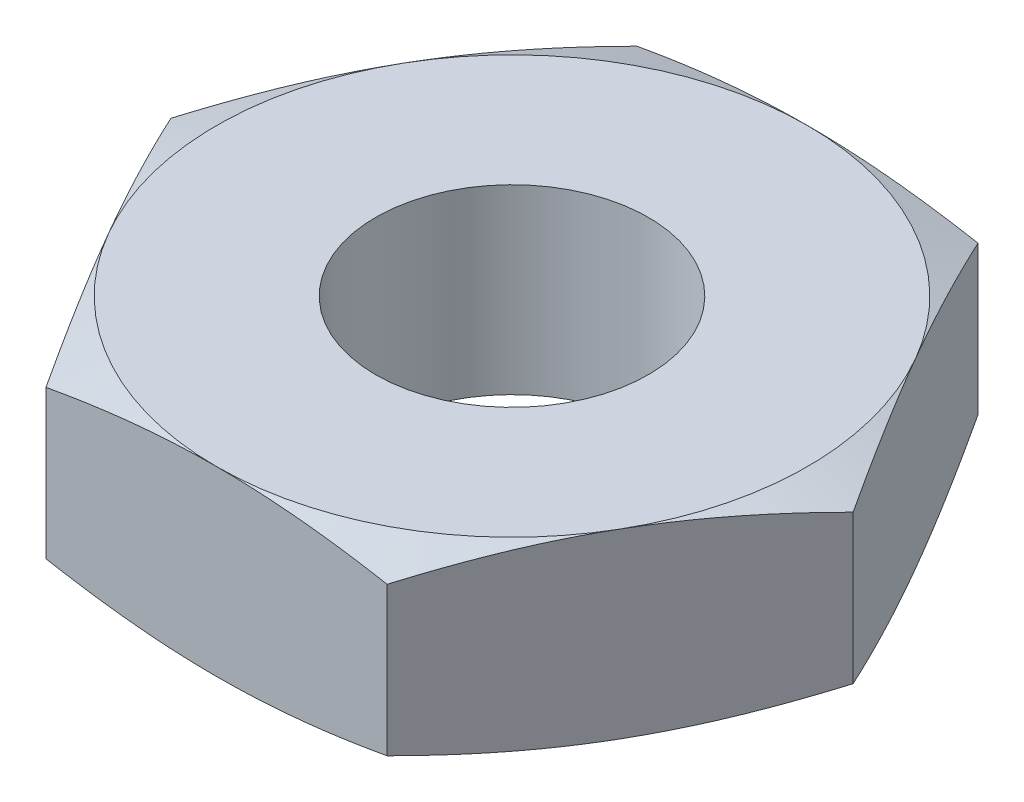
SolidWorks part; units mm, degrees
material "Plain Carbon Steel"
ref_plane "Front Plane" through (0, 0, 0) normal (0, 0, 1) x (1, 0, 0)
ref_plane "Top Plane" through (0, 0, 0) normal (0, 1, 0) x (1, 0, 0)
ref_plane "Right Plane" through (0, 0, 0) normal (1, 0, 0) x (0, 0, -1)
sketch "Hex Profile Sketch" plane through (0, 0, 0) normal (0, 1, 0) x (1, 0, 0)
  line L1 (15.0111, 0) -> (7.5056, 13)
  line L2 (7.5056, 13) -> (-7.5056, 13)
  line L3 (-7.5056, 13) -> (-15.0111, 0)
  line L4 (-15.0111, 0) -> (-7.5056, -13)
  line L5 (-7.5056, -13) -> (7.5056, -13)
  line L6 (7.5056, -13) -> (15.0111, 0)
  circle A0 centre (0, 0) radius 13 construction
  circle A1 centre (0, 0) radius 6
  dimension "D2" = 12
  dimension "D1" = 26
extrude "Hex Nut Body" add sketch "Hex Profile Sketch" along normal mid plane 8
sketch "Chamfer Circle Sketch" plane through (0, 4, 0) normal (0, 1, 0) x (1, 0, 0)
  circle A0 centre (0, 0) radius 13
  dimension "D1" = 26
extrude "Top Chamfer Cut 70deg" cut sketch "Chamfer Circle Sketch" against normal through all draft 70 flip side to cut
mirror "Bottom Chamfer Mirror" about plane through (0, 0, 0) normal (0, 1, 0) of "Top Chamfer Cut 70deg"
